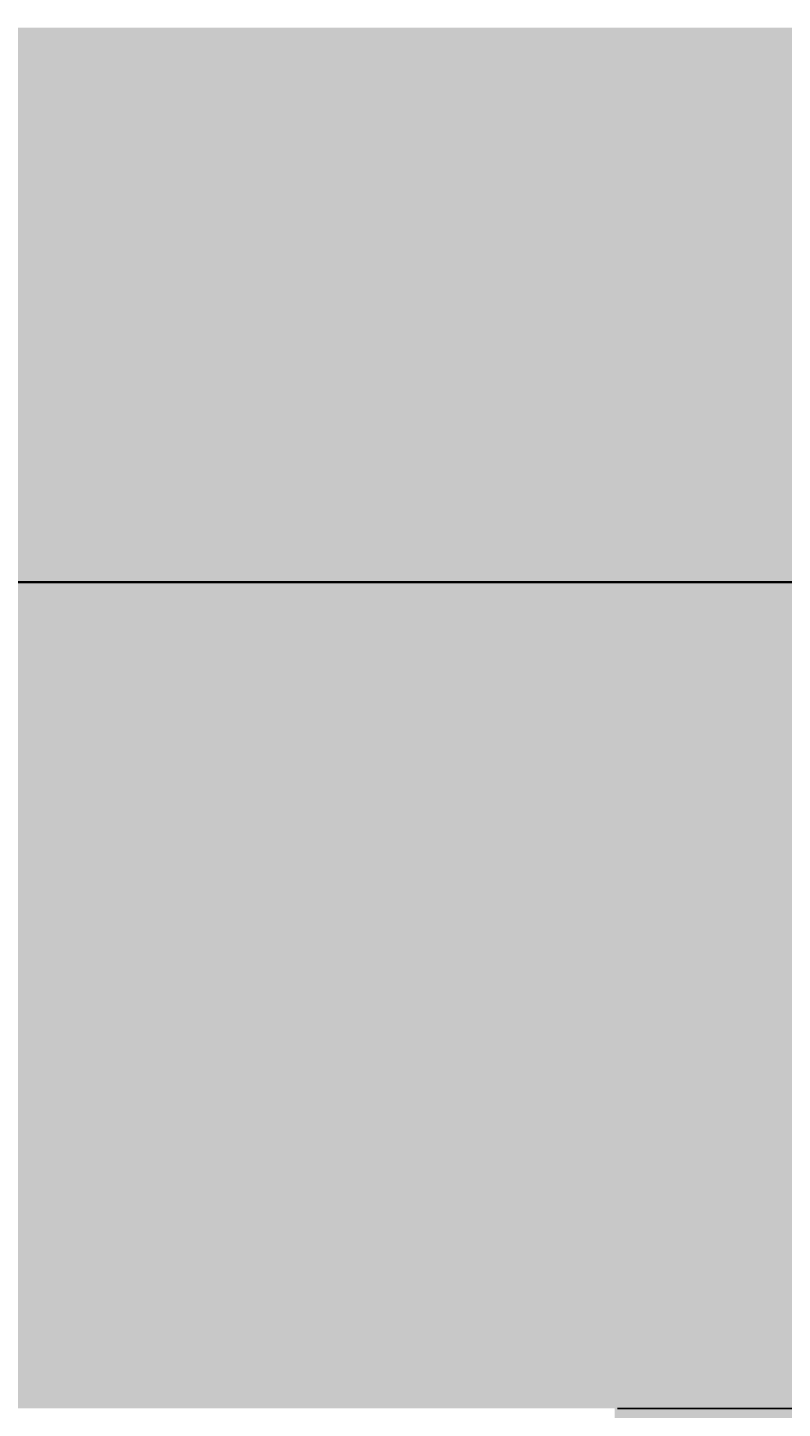
# Model space of a CAD drawing. Units: feet. Extents: x 2695 to 2912, y 795 to 1139.
# Tile 30 of 83: x 2825 to 2842, y 906 to 937. Entities that reach past the tile are written whole.
import ezdxf

# ---------------------------------------------------------------- set-up
doc = ezdxf.new("R2010")
doc.units = ezdxf.units.FT
for name, color, linetype, lineweight in [('A-ANNO-DIMS', 2, 'Continuous', 18), ('A-ELEV', 7, 'Continuous', 35), ('A-ELEV-PATT', 252, 'Continuous', 13)]:
    doc.layers.add(name, color=color, linetype=linetype, lineweight=lineweight)
doc.styles.get("Standard").update_dxf_attribs({"font": 'arial.ttf'})
doc.dimstyles.get("Standard").update_dxf_attribs({"dimtxt": 0.18, "dimasz": 0.18, "dimexe": 0.18, "dimexo": 0.0625, "dimgap": 0.09, "dimtad": 0, "dimtih": 1, "dimtoh": 1, "dimdec": 1, "dimzin": 0, "dimdsep": 46, "dimlunit": 3, "dimtxsty": 'Standard', "dimcen": 0.09, "dimadec": 0, "dimazin": 0, "dimtfac": 1, "dimtdec": 1, "dimtofl": 0, "dimtmove": 0, "dimatfit": 3, "dimfxl": 1, "dimtolj": 1, "dimtzin": 0, "dimarcsym": 0})

# ---------------------------------------------------------------- blocks, each defined once
blk = doc.blocks.new('*D14')
at = {"layer": 'A-ANNO-DIMS', "color": 0, "lineweight": -2, "transparency": 16777216}
for p, q in [((2838.439, 905.514), (2911.424, 905.514)), ((2911.244, 905.334), (2911.244, 890.368)), ((2911.244, 875.037), (2911.244, 890.004)), ((2758.214, 874.857), (2911.424, 874.857))]:
    blk.add_line(p, q, dxfattribs=at)
at = {"layer": 'A-ANNO-DIMS', "color": 0, "transparency": 16777216}
for points in [[(2911.214, 905.334), (2911.274, 905.334), (2911.244, 905.514)], [(2911.214, 875.037), (2911.274, 875.037), (2911.244, 874.857)]]:
    blk.add_solid(points, dxfattribs=at)
at = {"layer": 'Defpoints', "color": 0, "transparency": 16777216}
for p in [(2838.377, 905.514), (2911.244, 905.514), (2758.151, 874.857)]:
    blk.add_point(p, dxfattribs=at)
at = {"layer": 'A-ANNO-DIMS', "color": 0, "transparency": 16777216, "insert": (2911.244, 890.186), "char_height": 0.18, "attachment_point": 5}
blk.add_mtext('\\A1;30.66', dxfattribs=at)
blk = doc.blocks.new('*D15')
at = {"layer": 'A-ANNO-DIMS', "color": 0, "lineweight": -2, "transparency": 16777216}
for p, q in [((2890.699, 924.311), (2911.424, 924.311)), ((2911.244, 924.131), (2911.244, 915.094)), ((2911.244, 905.694), (2911.244, 914.731)), ((2838.439, 905.514), (2911.424, 905.514))]:
    blk.add_line(p, q, dxfattribs=at)
at = {"layer": 'A-ANNO-DIMS', "color": 0, "transparency": 16777216}
for points in [[(2911.214, 924.131), (2911.274, 924.131), (2911.244, 924.311)], [(2911.214, 905.694), (2911.274, 905.694), (2911.244, 905.514)]]:
    blk.add_solid(points, dxfattribs=at)
at = {"layer": 'Defpoints', "color": 0, "transparency": 16777216}
for p in [(2890.636, 924.311), (2911.244, 924.311), (2838.377, 905.514)]:
    blk.add_point(p, dxfattribs=at)
at = {"layer": 'A-ANNO-DIMS', "color": 0, "transparency": 16777216, "insert": (2911.244, 914.912), "char_height": 0.18, "attachment_point": 5}
blk.add_mtext('\\A1;18.796', dxfattribs=at)

msp = doc.modelspace()

# ---------------------------------------------------------------- hatches: boundary and pattern name
at = {"layer": 'A-ELEV-PATT'}
h = msp.add_hatch(color=256, dxfattribs=at)
h.set_gradient(color1=(255, 255, 255), tint=1)
h.paths.add_polyline_path([(2770.6361, 1122.9306), (2710.6361, 1122.9306), (2710.6361, 1118.4096), (2770.6361, 1118.4096)])
h.paths.add_polyline_path([(2890.6361, 1107.8588), (2770.6361, 1107.8588), (2770.6361, 1103.3378), (2890.6361, 1103.3378)])
h.paths.add_polyline_path([(2890.6361, 1062.9306), (2710.6361, 1062.9306), (2710.6361, 1056.9306), (2710.6361, 936.9306), (2710.6361, 924.3105), (2716.5358, 924.3105), (2890.6361, 924.3105), (2890.6361, 936.9306), (2715.8852, 936.9306), (2715.8852, 1050.3105), (2890.6361, 1050.3105)])
h.paths.add_polyline_path([(2716.5358, 924.3105), (2710.6361, 924.3105), (2710.6361, 810.9306), (2716.5358, 810.9306)])
h = msp.add_hatch(color=256, dxfattribs=at)
h.set_gradient(color1=(147, 149, 152), color2=(147, 149, 152), tint=1)
h.paths.add_polyline_path([(2770.6361, 1118.4096), (2710.6361, 1118.4096), (2710.6361, 1062.9306), (2770.6361, 1062.9306)])
h.paths.add_polyline_path([(2890.6361, 1103.3378), (2770.6361, 1103.3378), (2770.6361, 1062.9306), (2890.6361, 1062.9306)])
h.paths.add_polyline_path([(2730.7081, 1048.1052), (2755.1125, 1048.1052), (2755.1125, 936.9306), (2770.6361, 936.9306), (2770.6361, 1050.3105), (2715.8852, 1050.3105), (2715.8852, 936.9306), (2730.7081, 936.9306)])
h.paths.add_polyline_path([(2890.6361, 1050.3105), (2770.6361, 1050.3105), (2770.6361, 971.9673), (2778.0341, 971.9673), (2778.0341, 1020.8235), (2843.575, 1020.8235), (2843.575, 971.9673), (2890.6361, 971.9673)])
h.paths.add_polyline_path([(2888.1882, 970.7156), (2843.575, 970.7156), (2843.575, 964.8267), (2888.1882, 964.8267)])
h.paths.add_polyline_path([(2888.1882, 964.1328), (2843.575, 964.1328), (2843.575, 956.614), (2888.1882, 956.614)])
h.paths.add_polyline_path([(2888.1882, 955.9202), (2843.575, 955.9202), (2843.575, 949.2892), (2888.1882, 949.2892)])
h.paths.add_polyline_path([(2888.1882, 948.5954), (2843.575, 948.5954), (2843.575, 941.3507), (2888.1882, 941.3507)])
h.paths.add_polyline_path([(2888.1882, 940.6569), (2843.575, 940.6569), (2843.575, 936.9306), (2888.1882, 936.9306)])
h.paths.add_polyline_path([(2890.6361, 970.7156), (2888.9368, 970.7156), (2888.9368, 964.8267), (2890.6361, 964.8267)])
h.paths.add_polyline_path([(2890.6361, 964.1328), (2888.9368, 964.1328), (2888.9368, 956.614), (2890.6361, 956.614)])
h.paths.add_polyline_path([(2890.6361, 955.9202), (2888.9368, 955.9202), (2888.9368, 949.2892), (2890.6361, 949.2892)])
h.paths.add_polyline_path([(2890.6361, 940.6569), (2888.9368, 940.6569), (2888.9368, 936.9306), (2890.6361, 936.9306)])
h.paths.add_polyline_path([(2890.6361, 948.5954), (2888.9368, 948.5954), (2888.9368, 941.3507), (2890.6361, 941.3507)])
h.paths.add_polyline_path([(2772.5216, 970.7156), (2770.6361, 970.7156), (2770.6361, 964.8267), (2772.5216, 964.8267)])
h.paths.add_polyline_path([(2772.5216, 964.1328), (2770.6361, 964.1328), (2770.6361, 956.614), (2772.5216, 956.614)])
h.paths.add_polyline_path([(2772.5216, 955.9202), (2770.6361, 955.9202), (2770.6361, 949.2892), (2772.5216, 949.2892)])
h.paths.add_polyline_path([(2772.5216, 948.5954), (2770.6361, 948.5954), (2770.6361, 941.3507), (2772.5216, 941.3507)])
h.paths.add_polyline_path([(2772.5216, 940.6569), (2770.6361, 940.6569), (2770.6361, 936.9306), (2772.5216, 936.9306)])
h.paths.add_polyline_path([(2778.0341, 940.6569), (2773.2702, 940.6569), (2773.2702, 936.9306), (2778.0341, 936.9306)])
h.paths.add_polyline_path([(2778.0341, 970.7156), (2773.2702, 970.7156), (2773.2702, 964.8267), (2778.0341, 964.8267)])
h.paths.add_polyline_path([(2778.0341, 964.1328), (2773.2702, 964.1328), (2773.2702, 956.614), (2778.0341, 956.614)])
h.paths.add_polyline_path([(2778.0341, 955.9202), (2773.2702, 955.9202), (2773.2702, 949.2892), (2778.0341, 949.2892)])
h.paths.add_polyline_path([(2778.0341, 948.5954), (2773.2702, 948.5954), (2773.2702, 941.3507), (2778.0341, 941.3507)])
h.paths.add_polyline_path([(2810.0407, 940.6569), (2780.0341, 940.6569), (2780.0341, 936.9306), (2810.0407, 936.9306)])
h.paths.add_polyline_path([(2890.6361, 924.3105), (2770.6361, 924.3105), (2770.6361, 810.9306), (2773.5029, 810.9306), (2773.5029, 905.5143), (2805.9398, 905.5143), (2838.3767, 905.5143), (2838.3767, 810.9306), (2890.6361, 810.9306)])

# ---------------------------------------------------------------- linework, layer by layer
at = {"layer": 'A-ELEV'}
msp.add_lwpolyline([(2890.6361, 936.9306), (2890.6361, 924.3105), (2710.6361, 924.3105), (2710.6361, 936.9306)], dxfattribs=at)

# ---------------------------------------------------------------- dimensions: what is measured, and where the dimension line sits
at = {"layer": 'A-ANNO-DIMS'}
for base, p1, p2, override, picture, middle in [((2911.2444, 924.3105), (2838.3767, 905.5143), (2890.6361, 924.3105), {"dimdec": 3, "dimlfac": 1, "dimrnd": 0, "dimzin": 0, "dimdsep": 46, "dimlunit": 2}, '*D15', (2911.2444, 914.9124)), ((2911.2444, 905.5143), (2758.1515, 874.8571), (2838.3767, 905.5143), {"dimdec": 2, "dimlfac": 1, "dimrnd": 0, "dimzin": 0, "dimdsep": 46, "dimlunit": 2}, '*D14', (2911.2444, 890.1857))]:
    dim = msp.add_linear_dim(base=base, p1=p1, p2=p2, angle=90, dimstyle='Standard', override=override, dxfattribs=at)
    dim.commit()
    dim.dimension.update_dxf_attribs({"geometry": picture, "text_midpoint": middle})

doc.saveas('drawing.dxf')
